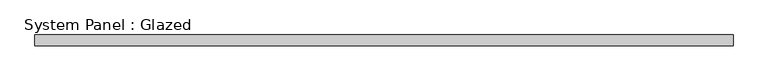
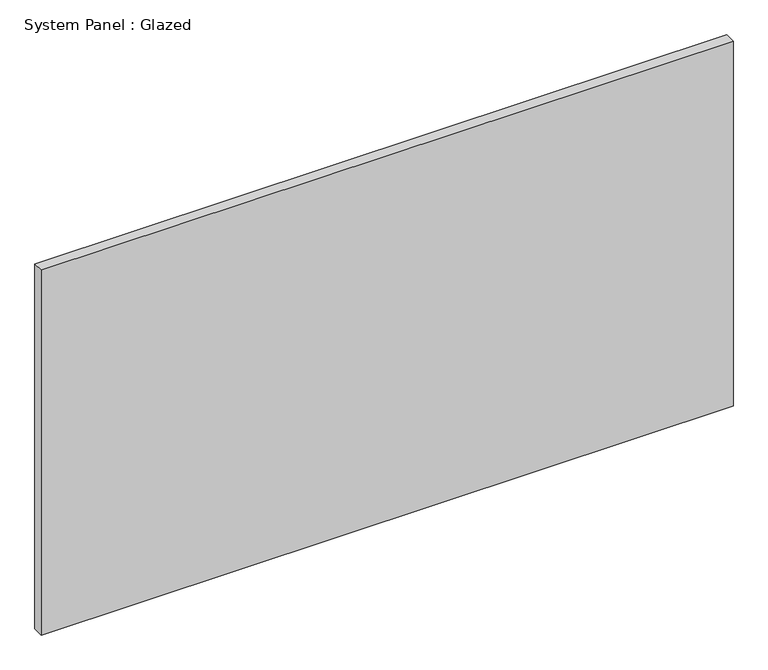
"""IFC4 building model written with IfcOpenShell, lengths in millimetres: plate geometry, System Panel : Glazed."""

from ifc_helpers import new_model, si_unit, origin, origin_with_axes, place, context, project, spatial, polyline, outline, extrude, source, transform, mapped, element, save


def system_panel_glazed_f6735284(model_context):
    return source(origin(), model_context, "Body", "SweptSolid", [
        extrude(outline(polyline([(819.2180043, 19.05), (-819.2180043, 19.05), (-819.2180043, 44.45), (819.2180043, 44.45), (819.2180043, 19.05)])), origin_with_axes(), (0.0, 0.0, 1.0), 914.4),
    ])


if __name__ == "__main__":
    model = new_model("IFC4")
    model_context = context("Model", 3, world=origin())
    ifc_project = project(units=[si_unit("LENGTHUNIT", "METRE", prefix="MILLI")], contexts=[model_context])
    site = spatial("IfcSite", under=ifc_project)
    building = spatial("IfcBuilding", under=site)
    placement = place(None, origin())
    system_panel_glazed_shape = system_panel_glazed_f6735284(model_context)
    element("IfcPlate", 1, ObjectType="System Panel : Glazed", at=placement, inside=building, context=model_context, shape_type="MappedRepresentation", body=[
        mapped(system_panel_glazed_shape, transform((0.0, 0.0, 0.0), x_axis=(1.0, 0.0, 0.0), y_axis=(0.0, 1.0, 0.0), z_axis=(0.0, 0.0, 1.0))),
    ])
    save(model, "model.ifc")

# Revit data of these elements
# Type "System Panel : Glazed"
#   Construction Type Id = "GSP4R"
#   Analytic Construction = "1/8 in Pilkington single glazing"
#   Visual Light Transmittance = 0.9
#   Solar Heat Gain Coefficient = 0.86
#   Heat Transfer Coefficient (U) = 1.18115 BTU/(h·ft²·°F)
# Element 1 (IfcPlate, "System Panel : Glazed")
#   Materials on its faces: "Glass"
# Materials
#   "Glass": class "Glass", colour RGB 0 128 192, transparency 0.75, Description = "Soda Lime Glass", Cost = 0
